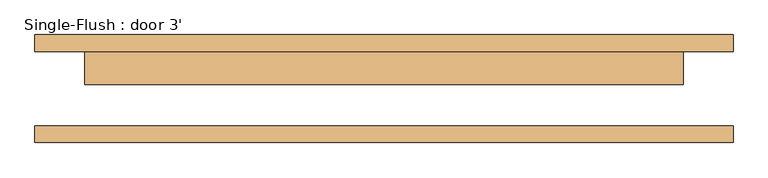
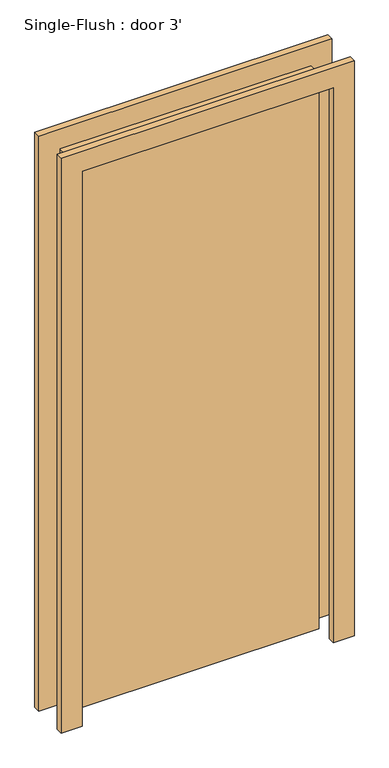
"""IFC4 building model written with IfcOpenShell, lengths in millimetres: door geometry, Single-Flush : door 3'."""

from ifc_helpers import new_model, si_unit, frame, origin, origin_with_axes, place, context, project, spatial, polyline, outline, extrude, source, transform, mapped, element, save


def single_flush_door_3_e5f9f3c4(model_context):
    return source(origin(), model_context, "Body", "SweptSolid", [
        extrude(outline(polyline([(2209.8, -533.4), (0.0, -533.4), (0.0, -457.2), (2133.6, -457.2), (2133.6, 457.2), (0.0, 457.2), (0.0, 533.4), (2209.8, 533.4), (2209.8, -533.4)])), frame((0.0, 57.15, 0.0), z_axis=(0.0, 1.0, 0.0), x_axis=(0.0, 0.0, 1.0)), (0.0, 0.0, 1.0), 25.4),
        extrude(outline(polyline([(2209.8, 533.4), (2209.8, -533.4), (0.0, -533.4), (0.0, -457.2), (2133.6, -457.2), (2133.6, 457.2), (0.0, 457.2), (0.0, 533.4), (2209.8, 533.4)])), frame((0.0, -82.55, 0.0), z_axis=(0.0, 1.0, 0.0), x_axis=(0.0, 0.0, 1.0)), (0.0, 0.0, 1.0), 25.4),
        extrude(outline(polyline([(457.2, 6.35), (-457.2, 6.35), (-457.2, 57.15), (457.2, 57.15), (457.2, 6.35)])), origin_with_axes(), (0.0, 0.0, 1.0), 2133.6),
    ])


if __name__ == "__main__":
    model = new_model("IFC4")
    model_context = context("Model", 3, world=origin())
    ifc_project = project(units=[si_unit("LENGTHUNIT", "METRE", prefix="MILLI")], contexts=[model_context])
    site = spatial("IfcSite", under=ifc_project)
    building = spatial("IfcBuilding", under=site)
    placement = place(None, origin())
    single_flush_door_3_shape = single_flush_door_3_e5f9f3c4(model_context)
    element("IfcDoor", 1, ObjectType="Single-Flush : door 3'", at=placement, inside=building, context=model_context, shape_type="MappedRepresentation", body=[
        mapped(single_flush_door_3_shape, transform((0.0, 0.0, 0.0), x_axis=(1.0, 0.0, 0.0), y_axis=(0.0, 1.0, 0.0), z_axis=(0.0, 0.0, 1.0))),
    ])
    save(model, "model.ifc")

# Revit data of these elements
# Type "Single-Flush : door 3'"
#   Type Mark = "8"
#   Construction Type Id = "MDOOR"
#   Assembly Code = "C1020"
#   Analytic Construction = "Metal"
#   Thickness = 0' - 2"
#   Heat Transfer Coefficient (U) = 0.651978 BTU/(h·ft²·°F)
#   Height = 7' - 0"
#   Trim Projection Ext = 0' - 1"
#   Trim Projection Int = 0' - 1"
#   Trim Width = 0' - 3"
#   Width = 3' - 0"
#   Define Thermal Properties by = 1
#   Door Material = Door - Panel
#   Frame Material = Door - Frame
#   Visual Light Transmittance = 0
#   Solar Heat Gain Coefficient = 0
#   Function = (empty or 0)
#   Wall Closure = (empty or 0)
# Element 1 (IfcDoor, "Single-Flush : door 3'")
#   Materials on its faces: "Door - Frame", "Door - Panel"
# Materials
#   "Door - Panel": class "Wood", colour RGB 210 159 95, transparency 0, Cost = 0
#   "Door - Frame": colour RGB 118 70 51, transparency 0, Cost = 0
